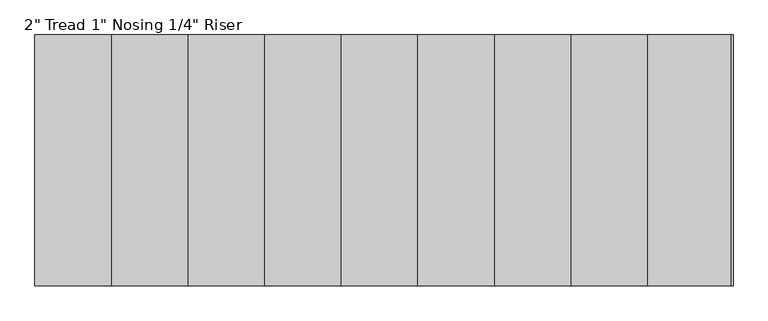
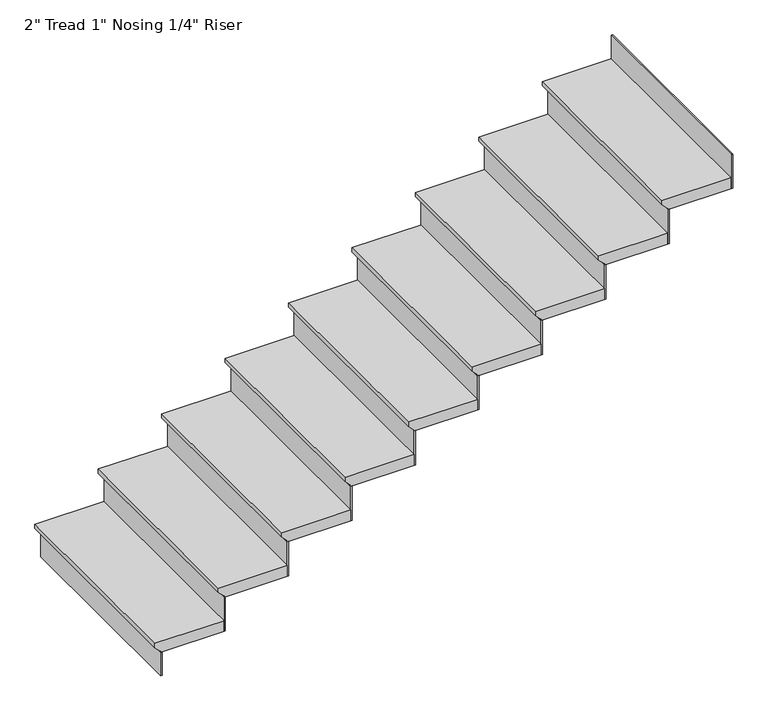
"""IFC4 building model written with IfcOpenShell, lengths in millimetres: stair flight geometry."""

from ifc_helpers import new_model, si_unit, origin, place, context, project, spatial, faceted_brep, source, transform, mapped, element, save


def stair_flight_a002e3d3(model_context):
    return source(origin(), model_context, "Body", "Brep", [
        faceted_brep([(-1591.1154463, -4737.3544725, 22543.77), (-1591.1154463, -4737.3544725, 22562.82), (-1591.1154463, -3822.9544725, 22562.82), (-1591.1154463, -3822.9544725, 22543.77), (-1565.7154463, -4737.3544725, 22518.37), (-1565.7154463, -3822.9544725, 22518.37), (-1286.3154463, -4737.3544725, 22562.82), (-1286.3154463, -3822.9544725, 22562.82), (-1565.7154463, -3822.9544725, 22512.02), (-1286.3154463, -3822.9544725, 22512.02), (-1286.3154463, -4737.3544725, 22512.02), (-1565.7154463, -4737.3544725, 22512.02)], [[[0, 1, 2, 3]], [[4, 0, 3, 5]], [[2, 1, 6, 7]], [[8, 9, 10, 11]], [[2, 7, 9, 8, 5, 3]], [[8, 11, 4, 5]], [[6, 1, 0, 4, 11, 10]], [[7, 6, 10, 9]]]),
        faceted_brep([(-1565.7154463, -4737.3544725, 22512.02), (-1565.7154463, -4737.3544725, 22402.8), (-1559.3654463, -4737.3544725, 22402.8), (-1559.3654463, -4737.3544725, 22512.02), (-1565.7154463, -3822.9544725, 22512.02), (-1559.3654463, -3822.9544725, 22512.02), (-1559.3654463, -3822.9544725, 22402.8), (-1565.7154463, -3822.9544725, 22402.8)], [[[0, 1, 2, 3]], [[4, 5, 6, 7]], [[1, 0, 4, 7]], [[2, 1, 7, 6]], [[3, 2, 6, 5]], [[0, 3, 5, 4]]]),
        faceted_brep([(-1286.3154463, -4737.3544725, 22672.04), (-1286.3154463, -4737.3544725, 22512.02), (-1279.9654463, -4737.3544725, 22512.02), (-1279.9654463, -4737.3544725, 22672.04), (-1286.3154463, -3822.9544725, 22672.04), (-1279.9654463, -3822.9544725, 22672.04), (-1279.9654463, -3822.9544725, 22512.02), (-1286.3154463, -3822.9544725, 22512.02)], [[[0, 1, 2, 3]], [[4, 5, 6, 7]], [[1, 0, 4, 7]], [[2, 1, 7, 6]], [[3, 2, 6, 5]], [[0, 3, 5, 4]]]),
        faceted_brep([(-1311.7154463, -3822.9544725, 22722.84), (-1311.7154463, -4737.3544725, 22722.84), (-1006.9154463, -4737.3544725, 22722.84), (-1006.9154463, -3822.9544725, 22722.84), (-1286.3154463, -3822.9544725, 22672.04), (-1006.9154463, -3822.9544725, 22672.04), (-1006.9154463, -4737.3544725, 22672.04), (-1286.3154463, -4737.3544725, 22672.04), (-1286.3154463, -3822.9544725, 22678.39), (-1311.7154463, -3822.9544725, 22703.79), (-1286.3154463, -4737.3544725, 22678.39), (-1311.7154463, -4737.3544725, 22703.79)], [[[0, 1, 2, 3]], [[4, 5, 6, 7]], [[0, 3, 5, 4, 8, 9]], [[4, 7, 10, 8]], [[2, 1, 11, 10, 7, 6]], [[3, 2, 6, 5]], [[11, 1, 0, 9]], [[10, 11, 9, 8]]]),
        faceted_brep([(-1006.9154463, -4737.3544725, 22832.06), (-1006.9154463, -4737.3544725, 22672.04), (-1000.5654463, -4737.3544725, 22672.04), (-1000.5654463, -4737.3544725, 22832.06), (-1006.9154463, -3822.9544725, 22832.06), (-1000.5654463, -3822.9544725, 22832.06), (-1000.5654463, -3822.9544725, 22672.04), (-1006.9154463, -3822.9544725, 22672.04)], [[[0, 1, 2, 3]], [[4, 5, 6, 7]], [[1, 0, 4, 7]], [[2, 1, 7, 6]], [[3, 2, 6, 5]], [[0, 3, 5, 4]]]),
        faceted_brep([(-1032.3154463, -3822.9544725, 22882.86), (-1032.3154463, -4737.3544725, 22882.86), (-727.5154463, -4737.3544725, 22882.86), (-727.5154463, -3822.9544725, 22882.86), (-1006.9154463, -3822.9544725, 22832.06), (-727.5154463, -3822.9544725, 22832.06), (-727.5154463, -4737.3544725, 22832.06), (-1006.9154463, -4737.3544725, 22832.06), (-1006.9154463, -3822.9544725, 22838.41), (-1032.3154463, -3822.9544725, 22863.81), (-1006.9154463, -4737.3544725, 22838.41), (-1032.3154463, -4737.3544725, 22863.81)], [[[0, 1, 2, 3]], [[4, 5, 6, 7]], [[0, 3, 5, 4, 8, 9]], [[4, 7, 10, 8]], [[2, 1, 11, 10, 7, 6]], [[3, 2, 6, 5]], [[11, 1, 0, 9]], [[10, 11, 9, 8]]]),
        faceted_brep([(-727.5154463, -4737.3544725, 22992.08), (-727.5154463, -4737.3544725, 22832.06), (-721.1654463, -4737.3544725, 22832.06), (-721.1654463, -4737.3544725, 22992.08), (-727.5154463, -3822.9544725, 22992.08), (-721.1654463, -3822.9544725, 22992.08), (-721.1654463, -3822.9544725, 22832.06), (-727.5154463, -3822.9544725, 22832.06)], [[[0, 1, 2, 3]], [[4, 5, 6, 7]], [[1, 0, 4, 7]], [[2, 1, 7, 6]], [[3, 2, 6, 5]], [[0, 3, 5, 4]]]),
        faceted_brep([(-752.9154463, -3822.9544725, 23042.88), (-752.9154463, -4737.3544725, 23042.88), (-448.1154463, -4737.3544725, 23042.88), (-448.1154463, -3822.9544725, 23042.88), (-727.5154463, -3822.9544725, 22992.08), (-448.1154463, -3822.9544725, 22992.08), (-448.1154463, -4737.3544725, 22992.08), (-727.5154463, -4737.3544725, 22992.08), (-727.5154463, -3822.9544725, 22998.43), (-752.9154463, -3822.9544725, 23023.83), (-727.5154463, -4737.3544725, 22998.43), (-752.9154463, -4737.3544725, 23023.83)], [[[0, 1, 2, 3]], [[4, 5, 6, 7]], [[0, 3, 5, 4, 8, 9]], [[4, 7, 10, 8]], [[2, 1, 11, 10, 7, 6]], [[3, 2, 6, 5]], [[11, 1, 0, 9]], [[10, 11, 9, 8]]]),
        faceted_brep([(-448.1154463, -4737.3544725, 23152.1), (-448.1154463, -4737.3544725, 22992.08), (-441.7654463, -4737.3544725, 22992.08), (-441.7654463, -4737.3544725, 23152.1), (-448.1154463, -3822.9544725, 23152.1), (-441.7654463, -3822.9544725, 23152.1), (-441.7654463, -3822.9544725, 22992.08), (-448.1154463, -3822.9544725, 22992.08)], [[[0, 1, 2, 3]], [[4, 5, 6, 7]], [[1, 0, 4, 7]], [[2, 1, 7, 6]], [[3, 2, 6, 5]], [[0, 3, 5, 4]]]),
        faceted_brep([(-473.5154463, -3822.9544725, 23202.9), (-473.5154463, -4737.3544725, 23202.9), (-168.7154463, -4737.3544725, 23202.9), (-168.7154463, -3822.9544725, 23202.9), (-448.1154463, -3822.9544725, 23152.1), (-168.7154463, -3822.9544725, 23152.1), (-168.7154463, -4737.3544725, 23152.1), (-448.1154463, -4737.3544725, 23152.1), (-448.1154463, -3822.9544725, 23158.45), (-473.5154463, -3822.9544725, 23183.85), (-448.1154463, -4737.3544725, 23158.45), (-473.5154463, -4737.3544725, 23183.85)], [[[0, 1, 2, 3]], [[4, 5, 6, 7]], [[0, 3, 5, 4, 8, 9]], [[4, 7, 10, 8]], [[2, 1, 11, 10, 7, 6]], [[3, 2, 6, 5]], [[11, 1, 0, 9]], [[10, 11, 9, 8]]]),
        faceted_brep([(-168.7154463, -4737.3544725, 23312.12), (-168.7154463, -4737.3544725, 23152.1), (-162.3654463, -4737.3544725, 23152.1), (-162.3654463, -4737.3544725, 23312.12), (-168.7154463, -3822.9544725, 23312.12), (-162.3654463, -3822.9544725, 23312.12), (-162.3654463, -3822.9544725, 23152.1), (-168.7154463, -3822.9544725, 23152.1)], [[[0, 1, 2, 3]], [[4, 5, 6, 7]], [[1, 0, 4, 7]], [[2, 1, 7, 6]], [[3, 2, 6, 5]], [[0, 3, 5, 4]]]),
        faceted_brep([(-194.1154463, -3822.9544725, 23362.92), (-194.1154463, -4737.3544725, 23362.92), (110.6845537, -4737.3544725, 23362.92), (110.6845537, -3822.9544725, 23362.92), (-168.7154463, -3822.9544725, 23312.12), (110.6845537, -3822.9544725, 23312.12), (110.6845537, -4737.3544725, 23312.12), (-168.7154463, -4737.3544725, 23312.12), (-168.7154463, -3822.9544725, 23318.47), (-194.1154463, -3822.9544725, 23343.87), (-168.7154463, -4737.3544725, 23318.47), (-194.1154463, -4737.3544725, 23343.87)], [[[0, 1, 2, 3]], [[4, 5, 6, 7]], [[0, 3, 5, 4, 8, 9]], [[4, 7, 10, 8]], [[2, 1, 11, 10, 7, 6]], [[3, 2, 6, 5]], [[11, 1, 0, 9]], [[10, 11, 9, 8]]]),
        faceted_brep([(110.6845537, -4737.3544725, 23472.14), (110.6845537, -4737.3544725, 23312.12), (117.0345537, -4737.3544725, 23312.12), (117.0345537, -4737.3544725, 23472.14), (110.6845537, -3822.9544725, 23472.14), (117.0345537, -3822.9544725, 23472.14), (117.0345537, -3822.9544725, 23312.12), (110.6845537, -3822.9544725, 23312.12)], [[[0, 1, 2, 3]], [[4, 5, 6, 7]], [[1, 0, 4, 7]], [[2, 1, 7, 6]], [[3, 2, 6, 5]], [[0, 3, 5, 4]]]),
        faceted_brep([(85.2845537, -3822.9544725, 23522.94), (85.2845537, -4737.3544725, 23522.94), (390.0845537, -4737.3544725, 23522.94), (390.0845537, -3822.9544725, 23522.94), (110.6845537, -3822.9544725, 23472.14), (390.0845537, -3822.9544725, 23472.14), (390.0845537, -4737.3544725, 23472.14), (110.6845537, -4737.3544725, 23472.14), (110.6845537, -3822.9544725, 23478.49), (85.2845537, -3822.9544725, 23503.89), (110.6845537, -4737.3544725, 23478.49), (85.2845537, -4737.3544725, 23503.89)], [[[0, 1, 2, 3]], [[4, 5, 6, 7]], [[0, 3, 5, 4, 8, 9]], [[4, 7, 10, 8]], [[2, 1, 11, 10, 7, 6]], [[3, 2, 6, 5]], [[11, 1, 0, 9]], [[10, 11, 9, 8]]]),
        faceted_brep([(390.0845537, -4737.3544725, 23632.16), (390.0845537, -4737.3544725, 23472.14), (396.4345537, -4737.3544725, 23472.14), (396.4345537, -4737.3544725, 23632.16), (390.0845537, -3822.9544725, 23632.16), (396.4345537, -3822.9544725, 23632.16), (396.4345537, -3822.9544725, 23472.14), (390.0845537, -3822.9544725, 23472.14)], [[[0, 1, 2, 3]], [[4, 5, 6, 7]], [[1, 0, 4, 7]], [[2, 1, 7, 6]], [[3, 2, 6, 5]], [[0, 3, 5, 4]]]),
        faceted_brep([(364.6845537, -3822.9544725, 23682.96), (364.6845537, -4737.3544725, 23682.96), (669.4845537, -4737.3544725, 23682.96), (669.4845537, -3822.9544725, 23682.96), (390.0845537, -3822.9544725, 23632.16), (669.4845537, -3822.9544725, 23632.16), (669.4845537, -4737.3544725, 23632.16), (390.0845537, -4737.3544725, 23632.16), (390.0845537, -3822.9544725, 23638.51), (364.6845537, -3822.9544725, 23663.91), (390.0845537, -4737.3544725, 23638.51), (364.6845537, -4737.3544725, 23663.91)], [[[0, 1, 2, 3]], [[4, 5, 6, 7]], [[0, 3, 5, 4, 8, 9]], [[4, 7, 10, 8]], [[2, 1, 11, 10, 7, 6]], [[3, 2, 6, 5]], [[11, 1, 0, 9]], [[10, 11, 9, 8]]]),
        faceted_brep([(948.8845537, -4737.3544725, 23952.2), (948.8845537, -4737.3544725, 23792.18), (955.2345537, -4737.3544725, 23792.18), (955.2345537, -4737.3544725, 23952.2), (948.8845537, -3822.9544725, 23952.2), (955.2345537, -3822.9544725, 23952.2), (955.2345537, -3822.9544725, 23792.18), (948.8845537, -3822.9544725, 23792.18)], [[[0, 1, 2, 3]], [[4, 5, 6, 7]], [[1, 0, 4, 7]], [[2, 1, 7, 6]], [[3, 2, 6, 5]], [[0, 3, 5, 4]]]),
        faceted_brep([(669.4845537, -4737.3544725, 23792.18), (669.4845537, -4737.3544725, 23632.16), (675.8345537, -4737.3544725, 23632.16), (675.8345537, -4737.3544725, 23792.18), (669.4845537, -3822.9544725, 23792.18), (675.8345537, -3822.9544725, 23792.18), (675.8345537, -3822.9544725, 23632.16), (669.4845537, -3822.9544725, 23632.16)], [[[0, 1, 2, 3]], [[4, 5, 6, 7]], [[1, 0, 4, 7]], [[2, 1, 7, 6]], [[3, 2, 6, 5]], [[0, 3, 5, 4]]]),
        faceted_brep([(948.8845537, -3822.9544725, 23842.98), (923.4845537, -3822.9544725, 23842.98), (644.0845537, -3822.9544725, 23842.98), (644.0845537, -4737.3544725, 23842.98), (948.8845537, -4737.3544725, 23842.98), (923.4845537, -3822.9544725, 23792.18), (948.8845537, -3822.9544725, 23792.18), (948.8845537, -4737.3544725, 23792.18), (669.4845537, -4737.3544725, 23792.18), (669.4845537, -3822.9544725, 23792.18), (669.4845537, -3822.9544725, 23798.53), (644.0845537, -3822.9544725, 23823.93), (669.4845537, -4737.3544725, 23798.53), (644.0845537, -4737.3544725, 23823.93)], [[[0, 1, 2, 3, 4]], [[5, 6, 7, 8, 9]], [[1, 0, 6, 5]], [[2, 1, 5, 9, 10, 11]], [[9, 8, 12, 10]], [[4, 3, 13, 12, 8, 7]], [[0, 4, 7, 6]], [[13, 3, 2, 11]], [[12, 13, 11, 10]]]),
    ])


if __name__ == "__main__":
    model = new_model("IFC4")
    model_context = context("Model", 3, world=origin())
    ifc_project = project(units=[si_unit("LENGTHUNIT", "METRE", prefix="MILLI")], contexts=[model_context])
    site = spatial("IfcSite", under=ifc_project)
    building = spatial("IfcBuilding", under=site)
    placement = place(None, origin())
    stair_flight_shape = stair_flight_a002e3d3(model_context)
    element("IfcStairFlight", 1, ObjectType="2\" Tread 1\" Nosing 1/4\" Riser", at=placement, inside=building, context=model_context, shape_type="MappedRepresentation", body=[
        mapped(stair_flight_shape, transform((0.0, 0.0, 0.0), x_axis=(1.0, 0.0, 0.0), y_axis=(0.0, 1.0, 0.0), z_axis=(0.0, 0.0, 1.0))),
    ])
    save(model, "model.ifc")
